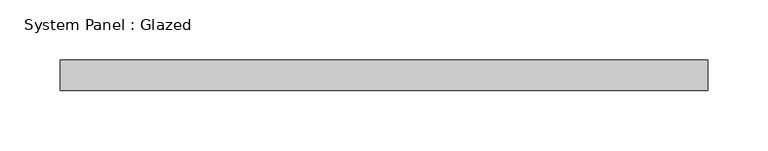
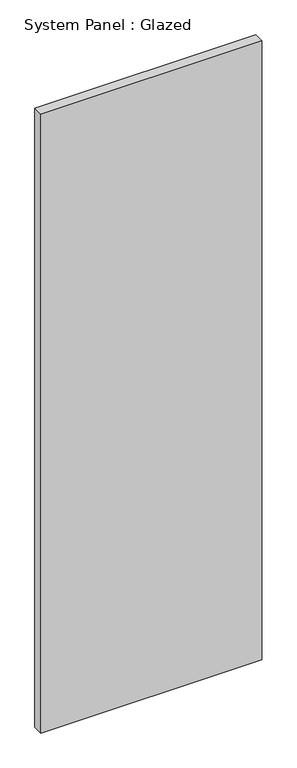
"""IFC4 building model written with IfcOpenShell, lengths in millimetres: plate geometry, System Panel : Glazed."""

from ifc_helpers import new_model, si_unit, origin, origin_with_axes, place, context, project, spatial, polyline, outline, extrude, source, transform, mapped, element, save


def system_panel_glazed_da8759c2(model_context):
    return source(origin(), model_context, "Body", "SweptSolid", [
        extrude(outline(polyline([(268.8166667, 19.05), (-268.8166667, 19.05), (-268.8166667, 44.45), (268.8166667, 44.45), (268.8166667, 19.05)])), origin_with_axes(), (0.0, 0.0, 1.0), 1591.7125392),
    ])


if __name__ == "__main__":
    model = new_model("IFC4")
    model_context = context("Model", 3, world=origin())
    ifc_project = project(units=[si_unit("LENGTHUNIT", "METRE", prefix="MILLI")], contexts=[model_context])
    site = spatial("IfcSite", under=ifc_project)
    building = spatial("IfcBuilding", under=site)
    placement = place(None, origin())
    system_panel_glazed_shape = system_panel_glazed_da8759c2(model_context)
    element("IfcPlate", 1, ObjectType="System Panel : Glazed", at=placement, inside=building, context=model_context, shape_type="MappedRepresentation", body=[
        mapped(system_panel_glazed_shape, transform((0.0, 0.0, 0.0), x_axis=(1.0, 0.0, 0.0), y_axis=(0.0, 1.0, 0.0), z_axis=(0.0, 0.0, 1.0))),
    ])
    save(model, "model.ifc")

# Revit data of these elements
# Type "System Panel : Glazed"
#   Construction Type Id = "GSP4R"
#   Analytic Construction = "1/8 in Pilkington single glazing"
#   Visual Light Transmittance = 0.9
#   Solar Heat Gain Coefficient = 0.86
#   Heat Transfer Coefficient (U) = 1.18115 BTU/(h·ft²·°F)
#   Define Thermal Properties by = 1
# Element 1 (IfcPlate, "System Panel : Glazed")
#   Materials on its faces: "Glass"
# Materials
#   "Glass": class "Glass", colour RGB 0 128 192, transparency 0.75, Description = "Soda Lime Glass", Cost = 0
